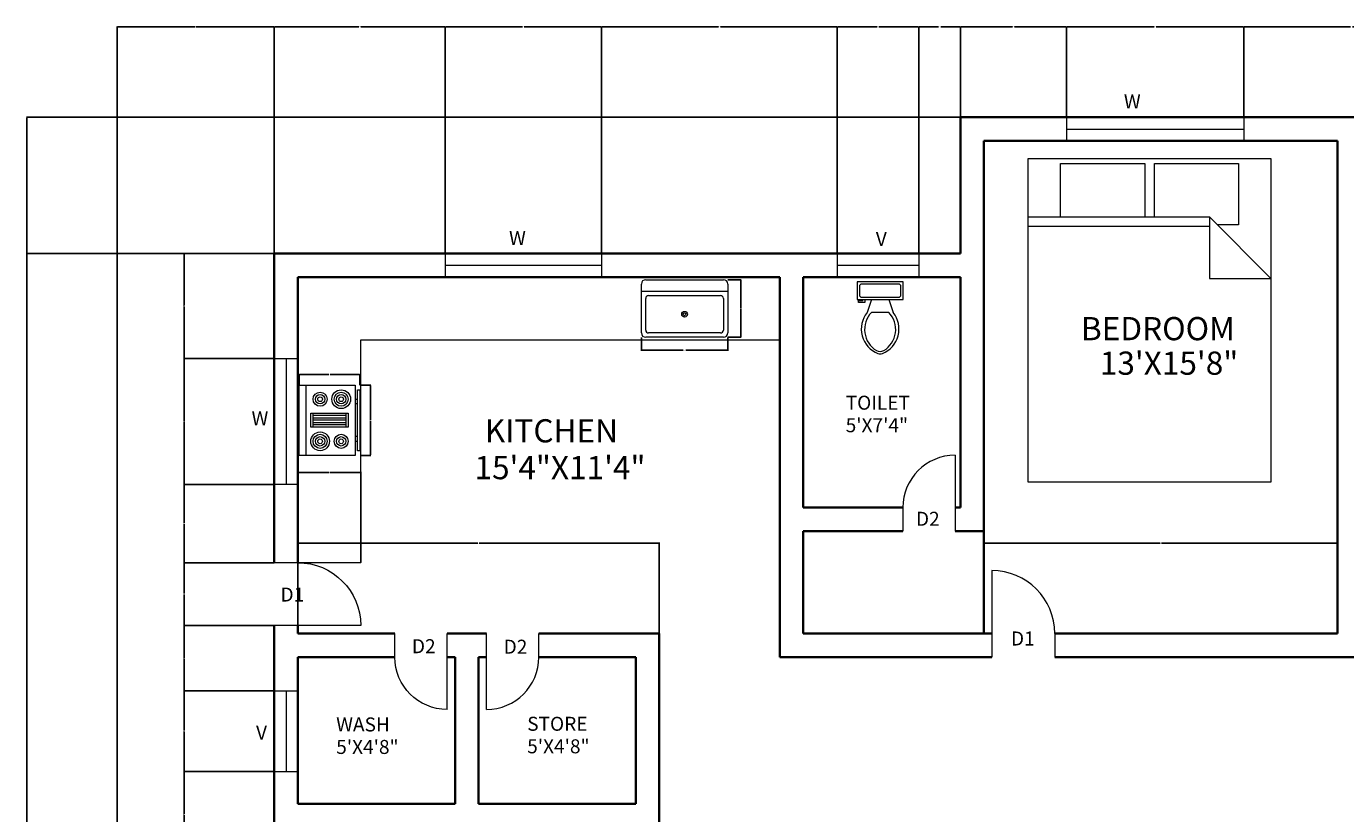
# Model space of a CAD drawing. Units: feet. Extents: x 1508 to 2265, y 1718 to 2421.
# Tile 3 of 4: x 1508 to 2012, y 2121 to 2421. Entities that reach past the tile are written whole.
import ezdxf

# ---------------------------------------------------------------- set-up
doc = ezdxf.new("R2010")
doc.units = ezdxf.units.FT
for name, color, linetype, lineweight in [('A-ANNO-DIMS', 2, 'Continuous', 18), ('A-ANNO-TEXT', 3, 'Continuous', 13), ('A-AREA-IDEN', 7, 'Continuous', 18), ('A-DOOR', 3, 'Continuous', 18), ('A-EQPM', 8, 'Continuous', 18), ('A-FLOR-CASE', 8, 'Continuous', 18), ('A-FLOR-FIXT', 9, 'Continuous', 18), ('A-FURN', 8, 'Continuous', 18), ('A-GLAZ', 4, 'Continuous', 18), ('A-WALL', 7, 'Continuous', 35), ('C-PROP', 7, 'Continuous', 25)]:
    doc.layers.add(name, color=color, linetype=linetype, lineweight=lineweight)
doc.styles.get("Standard").update_dxf_attribs({"font": 'arial.ttf'})
doc.dimstyles.get("Standard").update_dxf_attribs({"dimtxt": 0.18, "dimasz": 0.18, "dimexe": 0.18, "dimexo": 0.0625, "dimgap": 0.09, "dimtad": 0, "dimtih": 1, "dimtoh": 1, "dimdec": 4, "dimzin": 0, "dimdsep": 46, "dimtxsty": 'Standard', "dimcen": 0.09, "dimadec": 0, "dimazin": 0, "dimtfac": 1, "dimtdec": 4, "dimtofl": 0, "dimtmove": 0, "dimatfit": 3, "dimfxl": 1, "dimtolj": 1, "dimtzin": 0, "dimarcsym": 0})

# ---------------------------------------------------------------- blocks, each defined once
blk = doc.blocks.new('Toilet - top')
for p, q in [((9.5, -6), (9.5, -2)), ((-10, -8.5), (-8, -8.5)), ((-10, -9.5), (-10, -8.5)), ((-7, -9.5), (-10, -9.5)), ((-8, -8.5), (-8, -8)), ((-7, -8), (-7, -9.5)), ((-4, -8), (-6, -14)), ((4, -8), (6, -14)), ((4, -14), (-4, -14))]:
    blk.add_line(p, q)
blk.add_lwpolyline([(10.5, -8), (10.5, 0), (-10.5, 0), (-10.5, -8)], close=True)
for points in [[(-9.5, -2), (-9.5, -6)], [(8.5, -1), (-8.5, -1)], [(-8.5, -7), (8.5, -7)]]:
    blk.add_lwpolyline(points)
for centre, radius, start, end in [((-8.62, -1.88), 0.884, 81.8699, 188.1301), ((-8.62, -6.12), 0.884, 171.8699, 278.1301), ((8.62, -1.88), 0.884, 351.8699, 98.1301), ((8.62, -6.12), 0.884, 261.8699, 8.1301), ((3.52, -21.58), 12.17, 141.46911, 247.97143), ((4.2, -21.82), 11.33, 136.36773, 238.94682), ((-3.52, -21.58), 12.17, 292.02843, 38.53071), ((-4.2, -21.82), 11.33, 301.05301, 43.63209), ((0, -27.88), 4, 245.73182, 294.26817), ((0, -29), 4, 254.86053, 285.13947)]:
    blk.add_arc(centre, radius, start, end)
blk = doc.blocks.new('Range-Oven - 30 in top')
for p, q in [((0, -3), (30, -3)), ((12, -6), (18, -6)), ((13, -20), (13, -6)), ((14, -6), (14, -20)), ((15, -20), (15, -6)), ((16, -6), (16, -20)), ((17, -20), (17, -6)), ((18, -20), (12, -20)), ((6, -24), (6, -25)), ((8, -25), (8, -24)), ((22, -25), (22, -24)), ((24, -24), (24, -25))]:
    blk.add_line(p, q)
for points in [[(0, -24), (0, 0), (30, 0), (30, -24)], [(12, -21), (12, -5), (18, -5), (18, -21)], [(2, -26), (2, -25), (28, -25), (28, -26)]]:
    blk.add_lwpolyline(points, close=True)
for centre, radius in [((6, -9), 4), ((6, -9), 3), ((6, -9), 2), ((6, -9), 1), ((24, -9), 3), ((24, -9), 2), ((24, -9), 1), ((6, -18), 3), ((6, -18), 2), ((24, -18), 4), ((24, -18), 3), ((24, -18), 2), ((6, -18), 1), ((24, -18), 1)]:
    blk.add_circle(centre, radius)
blk = doc.blocks.new('Sink-single - 30 in top')
blk.add_line((-15, -3.999996), (15, -3.999996))
for points in [[(-13.5, 0), (13.5, 0)], [(-15, -18.499996), (-15, -1.5)], [(15, -1.5), (15, -18.499996)], [(-13.5, -17.499996), (-13.5, -6.499996)], [(-12.5, -5.499996), (12.5, -5.499996)], [(13.5, -6.499996), (13.5, -17.499996)], [(13.5, -19.999996), (-13.5, -19.999996)], [(12.5, -18.499996), (-12.5, -18.499996)]]:
    blk.add_lwpolyline(points)
for radius in [1, 0.5]:
    blk.add_circle((0, -11.999996), radius)
for centre, radius, start, end in [((-13.5, -1.5), 1.5, 90, 180), ((13.5, -1.5), 1.5, 0, 90), ((-12.5, -6.499996), 1, 90, 180), ((12.5, -6.499996), 1, 0, 90), ((-12.5, -17.499996), 1, 180, 270), ((12.5, -17.499996), 1, 270, 0), ((-13.5, -18.499996), 1.5, 180, 270), ((13.5, -18.499996), 1.5, 270, 0)]:
    blk.add_arc(centre, radius, start, end)
blk = doc.blocks.new('Bed - Queen')
for p, q in [((0, -80.00003), (0, 0)), ((0, 0), (59.99999, 0)), ((59.99999, 0), (59.99999, -80.00003)), ((7.99999, -1.2), (28.79998, -1.2)), ((7.99999, -14.4), (7.99999, -1.2)), ((28.79998, -1.2), (28.79998, -14.4)), ((31.19999, -1.2), (51.99999, -1.2)), ((31.19999, -14.4), (31.19999, -1.2)), ((51.99999, -1.2), (51.99999, -16.4)), ((0, -14.4), (44.8, -14.4)), ((59.99999, -29.6), (44.8, -14.4)), ((44.8, -14.4), (44.8, -29.6)), ((44.8, -16.8), (0, -16.8)), ((51.99999, -16.4), (46.79936, -16.4)), ((44.8, -29.6), (59.99999, -29.6)), ((59.99999, -80.00003), (0, -80.00003))]:
    blk.add_line(p, q)
blk = doc.blocks.new('DOOR-LEAF-24')
blk.add_line((0, 33), (0, 0))
blk.add_arc((0, 9), 24, 0, 90)
blk = doc.blocks.new('DOOR-LEAF-20')
blk.add_line((20, 29), (20, 0))
blk.add_arc((20, 9), 20, 90, 180)
blk = doc.blocks.new('*D27')
at = {"layer": 'A-ANNO-DIMS', "color": 0, "lineweight": -2, "transparency": 16777216}
for p, q in [((1635.54, 2284), (1639.67, 2284)), ((1639.49, 2283.82), (1639.49, 2270.79)), ((1639.49, 2257.39), (1639.49, 2270.42)), ((1635.54, 2257.21), (1639.67, 2257.21))]:
    blk.add_line(p, q, dxfattribs=at)
at = {"layer": 'A-ANNO-DIMS', "color": 0, "transparency": 16777216}
for points in [[(1639.46, 2283.82), (1639.52, 2283.82), (1639.49, 2284)], [(1639.46, 2257.39), (1639.52, 2257.39), (1639.49, 2257.21)]]:
    blk.add_solid(points, dxfattribs=at)
at = {"layer": 'Defpoints', "color": 0, "transparency": 16777216}
for p in [(1635.48, 2284), (1639.49, 2284), (1635.48, 2257.21)]:
    blk.add_point(p, dxfattribs=at)
at = {"layer": 'A-ANNO-DIMS', "color": 0, "transparency": 16777216, "insert": (1639.49, 2270.61), "char_height": 0.18, "attachment_point": 5}
blk.add_mtext('\\A1;RANGE 27', dxfattribs=at)
blk = doc.blocks.new('*D28')
at = {"layer": 'A-ANNO-DIMS', "color": 0, "lineweight": -2, "transparency": 16777216}
for p, q in [((1612.26, 2284.06), (1612.26, 2288.2)), ((1612.44, 2288.02), (1623.65, 2288.02)), ((1635.3, 2288.02), (1624.09, 2288.02)), ((1635.48, 2284.06), (1635.48, 2288.2))]:
    blk.add_line(p, q, dxfattribs=at)
at = {"layer": 'A-ANNO-DIMS', "color": 0, "transparency": 16777216}
for points in [[(1612.44, 2288.05), (1612.44, 2287.99), (1612.26, 2288.02)], [(1635.3, 2288.05), (1635.3, 2287.99), (1635.48, 2288.02)]]:
    blk.add_solid(points, dxfattribs=at)
at = {"layer": 'Defpoints', "color": 0, "transparency": 16777216}
for p in [(1612.26, 2288.02), (1612.26, 2284), (1635.48, 2284)]:
    blk.add_point(p, dxfattribs=at)
at = {"layer": 'A-ANNO-DIMS', "color": 0, "transparency": 16777216, "insert": (1623.87, 2288.02), "char_height": 0.18, "attachment_point": 5}
blk.add_mtext('\\A1;23', dxfattribs=at)
blk = doc.blocks.new('*D29')
at = {"layer": 'A-ANNO-DIMS', "color": 0, "lineweight": -2, "transparency": 16777216}
for p, q in [((1742.98, 2302.21), (1742.98, 2297.15)), ((1743.16, 2297.33), (1758.92, 2297.33)), ((1775.77, 2297.33), (1760.01, 2297.33)), ((1775.95, 2302.21), (1775.95, 2297.15))]:
    blk.add_line(p, q, dxfattribs=at)
at = {"layer": 'A-ANNO-DIMS', "color": 0, "transparency": 16777216}
for points in [[(1743.16, 2297.36), (1743.16, 2297.3), (1742.98, 2297.33)], [(1775.77, 2297.36), (1775.77, 2297.3), (1775.95, 2297.33)]]:
    blk.add_solid(points, dxfattribs=at)
at = {"layer": 'Defpoints', "color": 0, "transparency": 16777216}
for p in [(1742.98, 2302.28), (1775.95, 2302.28), (1775.95, 2297.33)]:
    blk.add_point(p, dxfattribs=at)
at = {"layer": 'A-ANNO-DIMS', "color": 0, "transparency": 16777216, "insert": (1759.46, 2297.33), "char_height": 0.18, "attachment_point": 5}
blk.add_mtext('\\A1;SINK 33', dxfattribs=at)
blk = doc.blocks.new('*D30')
at = {"layer": 'A-ANNO-DIMS', "color": 0, "lineweight": -2, "transparency": 16777216}
for p, q in [((1776.01, 2324.26), (1781.08, 2324.26)), ((1780.9, 2324.08), (1780.9, 2313.45)), ((1780.9, 2302.46), (1780.9, 2313.09)), ((1776.01, 2302.28), (1781.08, 2302.28))]:
    blk.add_line(p, q, dxfattribs=at)
at = {"layer": 'A-ANNO-DIMS', "color": 0, "transparency": 16777216}
for points in [[(1780.87, 2324.08), (1780.93, 2324.08), (1780.9, 2324.26)], [(1780.87, 2302.46), (1780.93, 2302.46), (1780.9, 2302.28)]]:
    blk.add_solid(points, dxfattribs=at)
at = {"layer": 'Defpoints', "color": 0, "transparency": 16777216}
for p in [(1775.95, 2324.26), (1780.9, 2324.26), (1775.95, 2302.28)]:
    blk.add_point(p, dxfattribs=at)
at = {"layer": 'A-ANNO-DIMS', "color": 0, "transparency": 16777216, "insert": (1780.9, 2313.27), "char_height": 0.18, "attachment_point": 5}
blk.add_mtext('\\A1;22', dxfattribs=at)
blk = doc.blocks.new('*D32')
at = {"layer": 'A-ANNO-DIMS', "color": 0, "lineweight": -2, "transparency": 16777216}
for p, q in [((1542.74, 2386.26), (1508.15, 2386.26)), ((1508.33, 2386.08), (1508.33, 2069.44)), ((1508.33, 1752.44), (1508.33, 2069.08)), ((1542.74, 1752.26), (1508.15, 1752.26))]:
    blk.add_line(p, q, dxfattribs=at)
at = {"layer": 'A-ANNO-DIMS', "color": 0, "transparency": 16777216}
for points in [[(1508.3, 2386.08), (1508.36, 2386.08), (1508.33, 2386.26)], [(1508.3, 1752.44), (1508.36, 1752.44), (1508.33, 1752.26)]]:
    blk.add_solid(points, dxfattribs=at)
at = {"layer": 'Defpoints', "color": 0, "transparency": 16777216}
for p in [(1508.33, 2386.26), (1542.8, 2386.26), (1542.8, 1752.26)]:
    blk.add_point(p, dxfattribs=at)
at = {"layer": 'A-ANNO-DIMS', "color": 0, "transparency": 16777216, "insert": (1508.33, 2069.26), "char_height": 0.18, "attachment_point": 5}
blk.add_mtext('\\A1;634', dxfattribs=at)
blk = doc.blocks.new('*D33')
at = {"layer": 'A-ANNO-DIMS', "color": 0, "lineweight": -2, "transparency": 16777216}
for p, q in [((1542.8, 2386.32), (1542.8, 2420.92)), ((1542.98, 2420.74), (1572.59, 2420.74)), ((1602.62, 2420.74), (1573.02, 2420.74)), ((1602.8, 2334.32), (1602.8, 2420.92))]:
    blk.add_line(p, q, dxfattribs=at)
at = {"layer": 'A-ANNO-DIMS', "color": 0, "transparency": 16777216}
for points in [[(1542.98, 2420.77), (1542.98, 2420.71), (1542.8, 2420.74)], [(1602.62, 2420.77), (1602.62, 2420.71), (1602.8, 2420.74)]]:
    blk.add_solid(points, dxfattribs=at)
at = {"layer": 'Defpoints', "color": 0, "transparency": 16777216}
for p in [(1602.8, 2420.74), (1542.8, 2386.26), (1602.8, 2334.26)]:
    blk.add_point(p, dxfattribs=at)
at = {"layer": 'A-ANNO-DIMS', "color": 0, "transparency": 16777216, "insert": (1572.8, 2420.74), "char_height": 0.18, "attachment_point": 5}
blk.add_mtext('\\A1;60', dxfattribs=at)
blk = doc.blocks.new('*D36')
at = {"layer": 'A-ANNO-DIMS', "color": 0, "lineweight": -2, "transparency": 16777216}
for p, q in [((1864.74, 2386.26), (1508.15, 2386.26)), ((1508.33, 2386.08), (1508.33, 2360.44)), ((1508.33, 2334.44), (1508.33, 2360.08)), ((1864.74, 2334.26), (1508.15, 2334.26))]:
    blk.add_line(p, q, dxfattribs=at)
at = {"layer": 'A-ANNO-DIMS', "color": 0, "transparency": 16777216}
for points in [[(1508.3, 2386.08), (1508.36, 2386.08), (1508.33, 2386.26)], [(1508.3, 2334.44), (1508.36, 2334.44), (1508.33, 2334.26)]]:
    blk.add_solid(points, dxfattribs=at)
at = {"layer": 'Defpoints', "color": 0, "transparency": 16777216}
for p in [(1508.33, 2386.26), (1864.8, 2386.26), (1864.8, 2334.26)]:
    blk.add_point(p, dxfattribs=at)
at = {"layer": 'A-ANNO-DIMS', "color": 0, "transparency": 16777216, "insert": (1508.33, 2360.26), "char_height": 0.18, "attachment_point": 5}
blk.add_mtext('\\A1;52', dxfattribs=at)
blk = doc.blocks.new('*D37')
at = {"layer": 'A-ANNO-DIMS', "color": 0, "lineweight": -2, "transparency": 16777216}
for p, q in [((1602.8, 2334.32), (1602.8, 2420.92)), ((1602.98, 2420.74), (1635.05, 2420.74)), ((1667.91, 2420.74), (1635.84, 2420.74)), ((1668.09, 2334.32), (1668.09, 2420.92))]:
    blk.add_line(p, q, dxfattribs=at)
at = {"layer": 'A-ANNO-DIMS', "color": 0, "transparency": 16777216}
for points in [[(1602.98, 2420.77), (1602.98, 2420.71), (1602.8, 2420.74)], [(1667.91, 2420.77), (1667.91, 2420.71), (1668.09, 2420.74)]]:
    blk.add_solid(points, dxfattribs=at)
at = {"layer": 'Defpoints', "color": 0, "transparency": 16777216}
for p in [(1668.09, 2420.74), (1602.8, 2334.26), (1668.09, 2334.26)]:
    blk.add_point(p, dxfattribs=at)
at = {"layer": 'A-ANNO-DIMS', "color": 0, "transparency": 16777216, "insert": (1635.45, 2420.74), "char_height": 0.18, "attachment_point": 5}
blk.add_mtext('\\A1;65.29', dxfattribs=at)
blk = doc.blocks.new('*D38')
at = {"layer": 'A-ANNO-DIMS', "color": 0, "lineweight": -2, "transparency": 16777216}
for p, q in [((1668.09, 2334.32), (1668.09, 2420.92)), ((1668.27, 2420.74), (1697.62, 2420.74)), ((1727.61, 2420.74), (1698.27, 2420.74)), ((1727.79, 2334.32), (1727.79, 2420.92))]:
    blk.add_line(p, q, dxfattribs=at)
at = {"layer": 'A-ANNO-DIMS', "color": 0, "transparency": 16777216}
for points in [[(1668.27, 2420.77), (1668.27, 2420.71), (1668.09, 2420.74)], [(1727.61, 2420.77), (1727.61, 2420.71), (1727.79, 2420.74)]]:
    blk.add_solid(points, dxfattribs=at)
at = {"layer": 'Defpoints', "color": 0, "transparency": 16777216}
for p in [(1727.79, 2420.74), (1668.09, 2334.26), (1727.79, 2334.26)]:
    blk.add_point(p, dxfattribs=at)
at = {"layer": 'A-ANNO-DIMS', "color": 0, "transparency": 16777216, "insert": (1697.94, 2420.74), "char_height": 0.18, "attachment_point": 5}
blk.add_mtext('\\A1;59.7', dxfattribs=at)
blk = doc.blocks.new('*D39')
at = {"layer": 'A-ANNO-DIMS', "color": 0, "lineweight": -2, "transparency": 16777216}
for p, q in [((1727.79, 2334.32), (1727.79, 2420.92)), ((1727.97, 2420.74), (1772.39, 2420.74)), ((1817.6, 2420.74), (1773.18, 2420.74)), ((1817.78, 2334.32), (1817.78, 2420.92))]:
    blk.add_line(p, q, dxfattribs=at)
at = {"layer": 'A-ANNO-DIMS', "color": 0, "transparency": 16777216}
for points in [[(1727.97, 2420.77), (1727.97, 2420.71), (1727.79, 2420.74)], [(1817.6, 2420.77), (1817.6, 2420.71), (1817.78, 2420.74)]]:
    blk.add_solid(points, dxfattribs=at)
at = {"layer": 'Defpoints', "color": 0, "transparency": 16777216}
for p in [(1817.78, 2420.74), (1727.79, 2334.26), (1817.78, 2334.26)]:
    blk.add_point(p, dxfattribs=at)
at = {"layer": 'A-ANNO-DIMS', "color": 0, "transparency": 16777216, "insert": (1772.79, 2420.74), "char_height": 0.18, "attachment_point": 5}
blk.add_mtext('\\A1;89.98', dxfattribs=at)
blk = doc.blocks.new('*D40')
at = {"layer": 'A-ANNO-DIMS', "color": 0, "lineweight": -2, "transparency": 16777216}
for p, q in [((1817.78, 2334.32), (1817.78, 2420.92)), ((1817.96, 2420.74), (1833.02, 2420.74)), ((1848.7, 2420.74), (1833.63, 2420.74)), ((1848.88, 2334.32), (1848.88, 2420.92))]:
    blk.add_line(p, q, dxfattribs=at)
at = {"layer": 'A-ANNO-DIMS', "color": 0, "transparency": 16777216}
for points in [[(1817.96, 2420.77), (1817.96, 2420.71), (1817.78, 2420.74)], [(1848.7, 2420.77), (1848.7, 2420.71), (1848.88, 2420.74)]]:
    blk.add_solid(points, dxfattribs=at)
at = {"layer": 'Defpoints', "color": 0, "transparency": 16777216}
for p in [(1848.88, 2420.74), (1817.78, 2334.26), (1848.88, 2334.26)]:
    blk.add_point(p, dxfattribs=at)
at = {"layer": 'A-ANNO-DIMS', "color": 0, "transparency": 16777216, "insert": (1833.33, 2420.74), "char_height": 0.18, "attachment_point": 5}
blk.add_mtext('\\A1;31.1', dxfattribs=at)
blk = doc.blocks.new('*D41')
at = {"layer": 'A-ANNO-DIMS', "color": 0, "lineweight": -2, "transparency": 16777216}
for p, q in [((1848.88, 2334.32), (1848.88, 2420.92)), ((1849.06, 2420.74), (1856.39, 2420.74)), ((1864.62, 2420.74), (1857.3, 2420.74)), ((1864.8, 2334.32), (1864.8, 2420.92))]:
    blk.add_line(p, q, dxfattribs=at)
at = {"layer": 'A-ANNO-DIMS', "color": 0, "transparency": 16777216}
for points in [[(1849.06, 2420.77), (1849.06, 2420.71), (1848.88, 2420.74)], [(1864.62, 2420.77), (1864.62, 2420.71), (1864.8, 2420.74)]]:
    blk.add_solid(points, dxfattribs=at)
at = {"layer": 'Defpoints', "color": 0, "transparency": 16777216}
for p in [(1864.8, 2420.74), (1848.88, 2334.26), (1864.8, 2334.26)]:
    blk.add_point(p, dxfattribs=at)
at = {"layer": 'A-ANNO-DIMS', "color": 0, "transparency": 16777216, "insert": (1856.84, 2420.74), "char_height": 0.18, "attachment_point": 5}
blk.add_mtext('\\A1;15.928', dxfattribs=at)
blk = doc.blocks.new('*D42')
at = {"layer": 'A-ANNO-DIMS', "color": 0, "lineweight": -2, "transparency": 16777216}
for p, q in [((1864.8, 2386.32), (1864.8, 2420.92)), ((1864.98, 2420.74), (1884.69, 2420.74)), ((1905.18, 2420.74), (1885.48, 2420.74)), ((1905.36, 2386.32), (1905.36, 2420.92))]:
    blk.add_line(p, q, dxfattribs=at)
at = {"layer": 'A-ANNO-DIMS', "color": 0, "transparency": 16777216}
for points in [[(1864.98, 2420.77), (1864.98, 2420.71), (1864.8, 2420.74)], [(1905.18, 2420.77), (1905.18, 2420.71), (1905.36, 2420.74)]]:
    blk.add_solid(points, dxfattribs=at)
at = {"layer": 'Defpoints', "color": 0, "transparency": 16777216}
for p in [(1905.36, 2420.74), (1864.8, 2386.26), (1905.36, 2386.26)]:
    blk.add_point(p, dxfattribs=at)
at = {"layer": 'A-ANNO-DIMS', "color": 0, "transparency": 16777216, "insert": (1885.08, 2420.74), "char_height": 0.18, "attachment_point": 5}
blk.add_mtext('\\A1;40.56', dxfattribs=at)
blk = doc.blocks.new('*D43')
at = {"layer": 'A-ANNO-DIMS', "color": 0, "lineweight": -2, "transparency": 16777216}
for p, q in [((1905.36, 2386.32), (1905.36, 2420.92)), ((1905.54, 2420.74), (1938.79, 2420.74)), ((1972.79, 2420.74), (1939.54, 2420.74)), ((1972.97, 2386.32), (1972.97, 2420.92))]:
    blk.add_line(p, q, dxfattribs=at)
at = {"layer": 'A-ANNO-DIMS', "color": 0, "transparency": 16777216}
for points in [[(1905.54, 2420.77), (1905.54, 2420.71), (1905.36, 2420.74)], [(1972.79, 2420.77), (1972.79, 2420.71), (1972.97, 2420.74)]]:
    blk.add_solid(points, dxfattribs=at)
at = {"layer": 'Defpoints', "color": 0, "transparency": 16777216}
for p in [(1972.97, 2420.74), (1905.36, 2386.26), (1972.97, 2386.26)]:
    blk.add_point(p, dxfattribs=at)
at = {"layer": 'A-ANNO-DIMS', "color": 0, "transparency": 16777216, "insert": (1939.17, 2420.74), "char_height": 0.18, "attachment_point": 5}
blk.add_mtext('\\A1;67.61', dxfattribs=at)
blk = doc.blocks.new('*D44')
at = {"layer": 'A-ANNO-DIMS', "color": 0, "lineweight": -2, "transparency": 16777216}
for p, q in [((1972.97, 2386.32), (1972.97, 2420.92)), ((1973.15, 2420.74), (2013.79, 2420.74)), ((2055.22, 2420.74), (2014.58, 2420.74)), ((2055.4, 2386.32), (2055.4, 2420.92))]:
    blk.add_line(p, q, dxfattribs=at)
at = {"layer": 'A-ANNO-DIMS', "color": 0, "transparency": 16777216}
for points in [[(1973.15, 2420.77), (1973.15, 2420.71), (1972.97, 2420.74)], [(2055.22, 2420.77), (2055.22, 2420.71), (2055.4, 2420.74)]]:
    blk.add_solid(points, dxfattribs=at)
at = {"layer": 'Defpoints', "color": 0, "transparency": 16777216}
for p in [(2055.4, 2420.74), (1972.97, 2386.26), (2055.4, 2386.26)]:
    blk.add_point(p, dxfattribs=at)
at = {"layer": 'A-ANNO-DIMS', "color": 0, "transparency": 16777216, "insert": (2014.19, 2420.74), "char_height": 0.18, "attachment_point": 5}
blk.add_mtext('\\A1;82.43', dxfattribs=at)
blk = doc.blocks.new('*D59')
at = {"layer": 'A-ANNO-DIMS', "color": 0, "lineweight": -2, "transparency": 16777216}
for p, q in [((1602.74, 2136.59), (1568.15, 2136.59)), ((1568.33, 2136.41), (1568.33, 2120.4)), ((1568.33, 2104.02), (1568.33, 2120.03)), ((1602.74, 2103.84), (1568.15, 2103.84))]:
    blk.add_line(p, q, dxfattribs=at)
at = {"layer": 'A-ANNO-DIMS', "color": 0, "transparency": 16777216}
for points in [[(1568.3, 2136.41), (1568.36, 2136.41), (1568.33, 2136.59)], [(1568.3, 2104.02), (1568.36, 2104.02), (1568.33, 2103.84)]]:
    blk.add_solid(points, dxfattribs=at)
at = {"layer": 'Defpoints', "color": 0, "transparency": 16777216}
for p in [(1568.33, 2136.59), (1602.8, 2136.59), (1602.8, 2103.84)]:
    blk.add_point(p, dxfattribs=at)
at = {"layer": 'A-ANNO-DIMS', "color": 0, "transparency": 16777216, "insert": (1568.33, 2120.22), "char_height": 0.18, "attachment_point": 5}
blk.add_mtext('\\A1;32.74', dxfattribs=at)
blk = doc.blocks.new('*D60')
at = {"layer": 'A-ANNO-DIMS', "color": 0, "lineweight": -2, "transparency": 16777216}
for p, q in [((1602.74, 2167.39), (1568.15, 2167.39)), ((1568.33, 2167.21), (1568.33, 2152.17)), ((1568.33, 2136.77), (1568.33, 2151.81)), ((1602.74, 2136.59), (1568.15, 2136.59))]:
    blk.add_line(p, q, dxfattribs=at)
at = {"layer": 'A-ANNO-DIMS', "color": 0, "transparency": 16777216}
for points in [[(1568.3, 2167.21), (1568.36, 2167.21), (1568.33, 2167.39)], [(1568.3, 2136.77), (1568.36, 2136.77), (1568.33, 2136.59)]]:
    blk.add_solid(points, dxfattribs=at)
at = {"layer": 'Defpoints', "color": 0, "transparency": 16777216}
for p in [(1568.33, 2167.39), (1602.8, 2167.39), (1602.8, 2136.59)]:
    blk.add_point(p, dxfattribs=at)
at = {"layer": 'A-ANNO-DIMS', "color": 0, "transparency": 16777216, "insert": (1568.33, 2151.99), "char_height": 0.18, "attachment_point": 5}
blk.add_mtext('\\A1;30.803', dxfattribs=at)
blk = doc.blocks.new('*D61')
at = {"layer": 'A-ANNO-DIMS', "color": 0, "lineweight": -2, "transparency": 16777216}
for p, q in [((1602.74, 2192.26), (1568.15, 2192.26)), ((1568.33, 2192.08), (1568.33, 2180.01)), ((1568.33, 2167.57), (1568.33, 2179.64)), ((1602.74, 2167.39), (1568.15, 2167.39))]:
    blk.add_line(p, q, dxfattribs=at)
at = {"layer": 'A-ANNO-DIMS', "color": 0, "transparency": 16777216}
for points in [[(1568.3, 2192.08), (1568.36, 2192.08), (1568.33, 2192.26)], [(1568.3, 2167.57), (1568.36, 2167.57), (1568.33, 2167.39)]]:
    blk.add_solid(points, dxfattribs=at)
at = {"layer": 'Defpoints', "color": 0, "transparency": 16777216}
for p in [(1568.33, 2192.26), (1602.8, 2192.26), (1602.8, 2167.39)]:
    blk.add_point(p, dxfattribs=at)
at = {"layer": 'A-ANNO-DIMS', "color": 0, "transparency": 16777216, "insert": (1568.33, 2179.83), "char_height": 0.18, "attachment_point": 5}
blk.add_mtext('\\A1;24.87', dxfattribs=at)
blk = doc.blocks.new('*D62')
at = {"layer": 'A-ANNO-DIMS', "color": 0, "lineweight": -2, "transparency": 16777216}
for p, q in [((1602.74, 2216.26), (1568.15, 2216.26)), ((1568.33, 2216.08), (1568.33, 2204.44)), ((1568.33, 2192.44), (1568.33, 2204.08)), ((1602.74, 2192.26), (1568.15, 2192.26))]:
    blk.add_line(p, q, dxfattribs=at)
at = {"layer": 'A-ANNO-DIMS', "color": 0, "transparency": 16777216}
for points in [[(1568.3, 2216.08), (1568.36, 2216.08), (1568.33, 2216.26)], [(1568.3, 2192.44), (1568.36, 2192.44), (1568.33, 2192.26)]]:
    blk.add_solid(points, dxfattribs=at)
at = {"layer": 'Defpoints', "color": 0, "transparency": 16777216}
for p in [(1568.33, 2216.26), (1602.8, 2216.26), (1602.8, 2192.26)]:
    blk.add_point(p, dxfattribs=at)
at = {"layer": 'A-ANNO-DIMS', "color": 0, "transparency": 16777216, "insert": (1568.33, 2204.26), "char_height": 0.18, "attachment_point": 5}
blk.add_mtext('\\A1;24', dxfattribs=at)
blk = doc.blocks.new('*D63')
at = {"layer": 'A-ANNO-DIMS', "color": 0, "lineweight": -2, "transparency": 16777216}
for p, q in [((1602.74, 2246.14), (1568.15, 2246.14)), ((1568.33, 2245.96), (1568.33, 2231.38)), ((1568.33, 2216.44), (1568.33, 2231.02)), ((1602.74, 2216.26), (1568.15, 2216.26))]:
    blk.add_line(p, q, dxfattribs=at)
at = {"layer": 'A-ANNO-DIMS', "color": 0, "transparency": 16777216}
for points in [[(1568.3, 2245.96), (1568.36, 2245.96), (1568.33, 2246.14)], [(1568.3, 2216.44), (1568.36, 2216.44), (1568.33, 2216.26)]]:
    blk.add_solid(points, dxfattribs=at)
at = {"layer": 'Defpoints', "color": 0, "transparency": 16777216}
for p in [(1568.33, 2246.14), (1602.8, 2246.14), (1602.8, 2216.26)]:
    blk.add_point(p, dxfattribs=at)
at = {"layer": 'A-ANNO-DIMS', "color": 0, "transparency": 16777216, "insert": (1568.33, 2231.2), "char_height": 0.18, "attachment_point": 5}
blk.add_mtext('\\A1;29.88', dxfattribs=at)
blk = doc.blocks.new('*D64')
at = {"layer": 'A-ANNO-DIMS', "color": 0, "lineweight": -2, "transparency": 16777216}
for p, q in [((1602.74, 2294.14), (1568.15, 2294.14)), ((1568.33, 2293.96), (1568.33, 2270.32)), ((1568.33, 2246.32), (1568.33, 2269.96)), ((1602.74, 2246.14), (1568.15, 2246.14))]:
    blk.add_line(p, q, dxfattribs=at)
at = {"layer": 'A-ANNO-DIMS', "color": 0, "transparency": 16777216}
for points in [[(1568.3, 2293.96), (1568.36, 2293.96), (1568.33, 2294.14)], [(1568.3, 2246.32), (1568.36, 2246.32), (1568.33, 2246.14)]]:
    blk.add_solid(points, dxfattribs=at)
at = {"layer": 'Defpoints', "color": 0, "transparency": 16777216}
for p in [(1568.33, 2294.14), (1602.8, 2294.14), (1602.8, 2246.14)]:
    blk.add_point(p, dxfattribs=at)
at = {"layer": 'A-ANNO-DIMS', "color": 0, "transparency": 16777216, "insert": (1568.33, 2270.14), "char_height": 0.18, "attachment_point": 5}
blk.add_mtext('\\A1;48', dxfattribs=at)
blk = doc.blocks.new('*D65')
at = {"layer": 'A-ANNO-DIMS', "color": 0, "lineweight": -2, "transparency": 16777216}
for p, q in [((1602.74, 2334.26), (1568.15, 2334.26)), ((1568.33, 2334.08), (1568.33, 2314.38)), ((1568.33, 2294.32), (1568.33, 2314.02)), ((1602.74, 2294.14), (1568.15, 2294.14))]:
    blk.add_line(p, q, dxfattribs=at)
at = {"layer": 'A-ANNO-DIMS', "color": 0, "transparency": 16777216}
for points in [[(1568.3, 2334.08), (1568.36, 2334.08), (1568.33, 2334.26)], [(1568.3, 2294.32), (1568.36, 2294.32), (1568.33, 2294.14)]]:
    blk.add_solid(points, dxfattribs=at)
at = {"layer": 'Defpoints', "color": 0, "transparency": 16777216}
for p in [(1568.33, 2334.26), (1602.8, 2334.26), (1602.8, 2294.14)]:
    blk.add_point(p, dxfattribs=at)
at = {"layer": 'A-ANNO-DIMS', "color": 0, "transparency": 16777216, "insert": (1568.33, 2314.2), "char_height": 0.18, "attachment_point": 5}
blk.add_mtext('\\A1;40.12', dxfattribs=at)
blk = doc.blocks.new('*D80')
at = {"layer": 'A-ANNO-DIMS', "color": 0, "lineweight": -2, "transparency": 16777216}
for p, q in [((1873.8, 2189.32), (1873.8, 2223.92)), ((1873.98, 2223.74), (1941.02, 2223.74)), ((2008.62, 2223.74), (1941.59, 2223.74)), ((2008.8, 2189.32), (2008.8, 2223.92))]:
    blk.add_line(p, q, dxfattribs=at)
at = {"layer": 'A-ANNO-DIMS', "color": 0, "transparency": 16777216}
for points in [[(1873.98, 2223.77), (1873.98, 2223.71), (1873.8, 2223.74)], [(2008.62, 2223.77), (2008.62, 2223.71), (2008.8, 2223.74)]]:
    blk.add_solid(points, dxfattribs=at)
at = {"layer": 'Defpoints', "color": 0, "transparency": 16777216}
for p in [(2008.8, 2223.74), (1873.8, 2189.26), (2008.8, 2189.26)]:
    blk.add_point(p, dxfattribs=at)
at = {"layer": 'A-ANNO-DIMS', "color": 0, "transparency": 16777216, "insert": (1941.3, 2223.74), "char_height": 0.18, "attachment_point": 5}
blk.add_mtext('\\A1;135', dxfattribs=at)
blk = doc.blocks.new('*D81')
at = {"layer": 'A-ANNO-DIMS', "color": 0, "lineweight": -2, "transparency": 16777216}
for p, q in [((1611.8, 2189.32), (1611.8, 2223.92)), ((1611.98, 2223.74), (1680.52, 2223.74)), ((1749.62, 2223.74), (1681.09, 2223.74)), ((1749.8, 2189.32), (1749.8, 2223.92))]:
    blk.add_line(p, q, dxfattribs=at)
at = {"layer": 'A-ANNO-DIMS', "color": 0, "transparency": 16777216}
for points in [[(1611.98, 2223.77), (1611.98, 2223.71), (1611.8, 2223.74)], [(1749.62, 2223.77), (1749.62, 2223.71), (1749.8, 2223.74)]]:
    blk.add_solid(points, dxfattribs=at)
at = {"layer": 'Defpoints', "color": 0, "transparency": 16777216}
for p in [(1749.8, 2223.74), (1611.8, 2189.26), (1749.8, 2189.26)]:
    blk.add_point(p, dxfattribs=at)
at = {"layer": 'A-ANNO-DIMS', "color": 0, "transparency": 16777216, "insert": (1680.8, 2223.74), "char_height": 0.18, "attachment_point": 5}
blk.add_mtext('\\A1;138', dxfattribs=at)
blk = doc.blocks.new('*D82')
at = {"layer": 'A-ANNO-DIMS', "color": 0, "lineweight": -2, "transparency": 16777216}
for p, q in [((1611.8, 2216.32), (1611.8, 2250.92)), ((1611.98, 2250.74), (1623.58, 2250.74)), ((1635.62, 2250.74), (1624.02, 2250.74)), ((1635.8, 2216.32), (1635.8, 2250.92))]:
    blk.add_line(p, q, dxfattribs=at)
at = {"layer": 'A-ANNO-DIMS', "color": 0, "transparency": 16777216}
for points in [[(1611.98, 2250.77), (1611.98, 2250.71), (1611.8, 2250.74)], [(1635.62, 2250.77), (1635.62, 2250.71), (1635.8, 2250.74)]]:
    blk.add_solid(points, dxfattribs=at)
at = {"layer": 'Defpoints', "color": 0, "transparency": 16777216}
for p in [(1635.8, 2250.74), (1611.8, 2216.26), (1635.8, 2216.26)]:
    blk.add_point(p, dxfattribs=at)
at = {"layer": 'A-ANNO-DIMS', "color": 0, "transparency": 16777216, "insert": (1623.8, 2250.74), "char_height": 0.18, "attachment_point": 5}
blk.add_mtext('\\A1;24', dxfattribs=at)

msp = doc.modelspace()

# ---------------------------------------------------------------- linework, layer by layer
at = {"layer": 'A-DOOR'}
for p, q in [((1842.8049, 2237.2608), (1842.8049, 2228.2608)), ((1648.8049, 2180.2608), (1648.8049, 2189.2608)), ((1703.8049, 2180.2608), (1703.8049, 2189.2608)), ((1900.8049, 2189.2608), (1900.8049, 2180.2608))]:
    msp.add_line(p, q, dxfattribs=at)
at = {"layer": 'A-FLOR-CASE'}
for p, q in [((1635.8049, 2301.2608), (1795.8049, 2301.2608)), ((1635.8049, 2216.2608), (1635.8049, 2301.2608)), ((1635.8049, 2216.2608), (1602.8049, 2216.2608))]:
    msp.add_line(p, q, dxfattribs=at)
at = {"layer": 'A-GLAZ'}
for p, q in [((1905.3626, 2386.2608), (1905.3626, 2377.2608)), ((1972.9732, 2386.2608), (1972.9732, 2377.2608)), ((1905.3626, 2381.7608), (1972.9732, 2381.7608)), ((1668.0907, 2334.2608), (1668.0907, 2325.2608)), ((1727.7948, 2334.2608), (1727.7948, 2325.2608)), ((1817.7791, 2334.2608), (1817.7791, 2325.2608)), ((1848.8765, 2334.2608), (1848.8765, 2325.2608)), ((1668.0907, 2329.7608), (1727.7948, 2329.7608)), ((1817.7791, 2329.7608), (1848.8765, 2329.7608)), ((1602.8049, 2294.1395), (1611.8049, 2294.1395)), ((1607.3049, 2294.1395), (1607.3049, 2246.1395)), ((1611.8049, 2246.1395), (1602.8049, 2246.1395)), ((1602.8049, 2167.3913), (1611.8049, 2167.3913)), ((1607.3049, 2167.3913), (1607.3049, 2136.588)), ((1602.8049, 2136.588), (1611.8049, 2136.588))]:
    msp.add_line(p, q, dxfattribs=at)
at = {"layer": 'A-WALL'}
for p, q in [((2170.8049, 2386.2608), (1864.8049, 2386.2608)), ((1864.8049, 2334.2608), (1864.8049, 2386.2608)), ((1873.8049, 2377.2608), (1873.8049, 2189.2608)), ((2008.8049, 2377.2608), (1873.8049, 2377.2608)), ((2008.8049, 2377.2608), (2008.8049, 2189.2608)), ((1602.8049, 2334.2608), (1864.8049, 2334.2608)), ((1602.8049, 2334.2608), (1602.8049, 2216.2608)), ((1602.8049, 2216.2608), (1602.8049, 2334.2608)), ((1804.8049, 2334.2608), (1864.8049, 2334.2608)), ((1611.8049, 2325.2608), (1795.8049, 2325.2608)), ((1611.8049, 2216.2608), (1611.8049, 2325.2608)), ((1795.8049, 2325.2608), (1795.8049, 2180.2608)), ((1804.8049, 2325.2608), (1804.8049, 2237.2608)), ((1804.8049, 2325.2608), (1864.8049, 2325.2608)), ((1864.8049, 2325.2608), (1864.8049, 2237.2608)), ((1842.8049, 2237.2608), (1804.8049, 2237.2608)), ((1864.8049, 2237.2608), (1862.8049, 2237.2608)), ((1804.8049, 2228.2608), (1804.8049, 2189.2608)), ((1842.8049, 2228.2608), (1804.8049, 2228.2608)), ((1873.8049, 2228.2608), (1862.8049, 2228.2608)), ((1602.8049, 2189.2608), (1602.8049, 2192.2608)), ((1602.8049, 2192.2608), (1602.8049, 1752.2608)), ((1611.8049, 2189.2608), (1611.8049, 2192.2608)), ((1648.8049, 2189.2608), (1611.8049, 2189.2608)), ((1683.8049, 2189.2608), (1668.8049, 2189.2608)), ((1749.8049, 2189.2608), (1703.8049, 2189.2608)), ((1749.8049, 2189.2608), (1749.8049, 2082.2608)), ((1804.8049, 2189.2608), (1873.8049, 2189.2608)), ((1873.8049, 2189.2608), (1876.8049, 2189.2608)), ((1900.8049, 2189.2608), (2008.8049, 2189.2608)), ((1611.8049, 2180.2608), (1611.8049, 2124.2608)), ((1648.8049, 2180.2608), (1611.8049, 2180.2608)), ((1671.8049, 2180.2608), (1668.8049, 2180.2608)), ((1671.8049, 2124.2608), (1671.8049, 2180.2608)), ((1680.8049, 2124.2608), (1680.8049, 2180.2608)), ((1683.8049, 2180.2608), (1680.8049, 2180.2608)), ((1740.8049, 2180.2608), (1703.8049, 2180.2608)), ((1740.8049, 2124.2608), (1740.8049, 2180.2608)), ((1749.8049, 2124.2608), (1749.8049, 2180.2608)), ((1795.8049, 2180.2608), (1873.8049, 2180.2608)), ((1873.8049, 2180.2608), (1876.8049, 2180.2608)), ((1900.8049, 2180.2608), (2020.8049, 2180.2608)), ((1611.8049, 2124.2608), (1671.8049, 2124.2608)), ((1680.8049, 2124.2608), (1740.8049, 2124.2608))]:
    msp.add_line(p, q, dxfattribs=at)
at = {"layer": 'C-PROP'}
for p, q in [((1542.8049, 2386.2608), (1542.8049, 1752.2608)), ((1550.6008, 2386.2608), (1542.8049, 2386.2608)), ((1864.8049, 2386.2608), (1550.6008, 2386.2608))]:
    msp.add_line(p, q, dxfattribs=at)

# ---------------------------------------------------------------- block references
at = {"layer": 'A-DOOR'}
for name, p in [('DOOR-LEAF-20', (1842.805, 2228.261)), ('DOOR-LEAF-24', (1876.805, 2180.261))]:
    msp.add_blockref(name, p, dxfattribs=at)
at = {"layer": 'A-DOOR', "extrusion": (0, 0, -1), "zscale": -1}
for name, p, rotation in [('DOOR-LEAF-24', (-1602.8051, 2192.2609), 90.00000000000003), ('DOOR-LEAF-20', (-1648.805, 2189.2605), 180)]:
    msp.add_blockref(name, p, dxfattribs=dict(at, rotation=rotation))
at = {"layer": 'A-DOOR', "rotation": 180}
msp.add_blockref('DOOR-LEAF-20', (1703.8048, 2189.2605), dxfattribs=at)
at = {"layer": 'A-EQPM', "xscale": 0.8928425473351428, "yscale": 0.8928425473351428, "zscale": 0.8928425473351428, "rotation": 90}
msp.add_blockref('Range-Oven - 30 in top', (1612.2625, 2257.2143), dxfattribs=at)
at = {"layer": 'A-FLOR-FIXT'}
for name, p, xscale, yscale, zscale in [('Sink-single - 30 in top', (1759.4627, 2324.2589), 1.0991701712874, 1.0991701712874, 1.0991701712874), ('Toilet - top', (1834.1521, 2323.3927), 0.8315942650714294, 0.8315942650714294, 0.8315942650714294)]:
    msp.add_blockref(name, p, dxfattribs=dict(at, xscale=xscale, yscale=yscale, zscale=zscale))
at = {"layer": 'A-FURN', "xscale": 1.544203597856591, "yscale": 1.544203597856591, "zscale": 1.544203597856591}
msp.add_blockref('Bed - Queen', (1890.7332, 2370.4676), dxfattribs=at)

# ---------------------------------------------------------------- texts
at = {"layer": 'A-ANNO-TEXT'}
for s, height, p in [('W', 5.3453, (1927.2349, 2389.5868)), ('W', 5.3453, (1692.4384, 2337.4808)), ('V', 5.3453, (1832.4981, 2337.1552)), ('W', 5.3453, (1594.1134, 2268.7068)), ('D2', 5.34528, (1847.8152, 2230.3335)), ('D1', 5.34528, (1605.1638, 2201.4268)), ('D2', 5.34528, (1655.3347, 2181.716)), ('D2', 5.34528, (1690.3657, 2181.5194)), ('D1', 5.34528, (1884.1045, 2184.6556)), ('V', 5.3453, (1595.8231, 2148.7734))]:
    msp.add_text(s, height=height, dxfattribs=at).set_placement(p)
at = {"layer": 'A-AREA-IDEN'}
for s, height, p in [('BEDROOM', 8.85057, (1910.8309, 2301.1506)), ('13\'X15\'8"', 8.85057, (1918.0425, 2287.9785)), ('TOILET', 5.34528, (1820.9878, 2274.6427)), ('KITCHEN', 8.85057, (1683.1683, 2262.159)), ('5\'X7\'4"', 5.34528, (1820.9878, 2266.056)), ('15\'4"X11\'4"', 8.850571, (1679.2457, 2248.1195)), ('WASH', 5.34528, (1626.4303, 2151.8569)), ('STORE', 5.34528, (1699.3645, 2152.1031)), ('5\'X4\'8"', 5.34528, (1626.4303, 2143.2702)), ('5\'X4\'8"', 5.34528, (1699.3645, 2143.5164))]:
    msp.add_text(s, height=height, dxfattribs=at).set_placement(p)

# ---------------------------------------------------------------- dimensions: what is measured, and where the dimension line sits
at = {"layer": 'A-ANNO-DIMS'}
for base, p1, p2, override, picture, middle in [((1602.8049, 2420.7358), (1542.8049, 2386.2608), (1602.8049, 2334.2608), {"dimdec": 0, "dimlfac": 1, "dimrnd": 0, "dimzin": 0, "dimdsep": 46, "dimlunit": 2}, '*D33', (1572.8049, 2420.7358)), ((1668.0907, 2420.7358), (1602.8049, 2334.2608), (1668.0907, 2334.2608), {"dimdec": 2, "dimlfac": 1, "dimrnd": 0, "dimzin": 0, "dimdsep": 46, "dimlunit": 2}, '*D37', (1635.4478, 2420.7358)), ((1727.7948, 2420.7358), (1668.0907, 2334.2608), (1727.7948, 2334.2608), {"dimdec": 1, "dimlfac": 1, "dimrnd": 0, "dimzin": 0, "dimdsep": 46, "dimlunit": 2}, '*D38', (1697.9427, 2420.7358)), ((1817.7791, 2420.7358), (1727.7948, 2334.2608), (1817.7791, 2334.2608), {"dimdec": 2, "dimlfac": 1, "dimrnd": 0, "dimzin": 0, "dimdsep": 46, "dimlunit": 2}, '*D39', (1772.7869, 2420.7358)), ((1848.8765, 2420.7358), (1817.7791, 2334.2608), (1848.8765, 2334.2608), {"dimdec": 1, "dimlfac": 1, "dimrnd": 0, "dimzin": 0, "dimdsep": 46, "dimlunit": 2}, '*D40', (1833.3278, 2420.7358)), ((1864.8049, 2420.7358), (1848.8765, 2334.2608), (1864.8049, 2334.2608), {"dimdec": 3, "dimlfac": 1, "dimrnd": 0, "dimzin": 0, "dimdsep": 46, "dimlunit": 2}, '*D41', (1856.8407, 2420.7358)), ((1905.3626, 2420.7358), (1864.8049, 2386.2608), (1905.3626, 2386.2608), {"dimdec": 2, "dimlfac": 1, "dimrnd": 0, "dimzin": 0, "dimdsep": 46, "dimlunit": 2}, '*D42', (1885.0837, 2420.7358)), ((1972.9732, 2420.7358), (1905.3626, 2386.2608), (1972.9732, 2386.2608), {"dimdec": 2, "dimlfac": 1, "dimrnd": 0, "dimzin": 0, "dimdsep": 46, "dimlunit": 2}, '*D43', (1939.1679, 2420.7358)), ((2055.3983, 2420.7358), (1972.9732, 2386.2608), (2055.3983, 2386.2608), {"dimdec": 2, "dimlfac": 1, "dimrnd": 0, "dimzin": 0, "dimdsep": 46, "dimlunit": 2}, '*D44', (2014.1857, 2420.7358)), ((1635.8049, 2250.7358), (1611.8049, 2216.2608), (1635.8049, 2216.2608), {"dimdec": 0, "dimlfac": 1, "dimrnd": 0, "dimzin": 0, "dimdsep": 46, "dimlunit": 2}, '*D82', (1623.8049, 2250.7358)), ((1749.8049, 2223.7358), (1611.8049, 2189.2608), (1749.8049, 2189.2608), {"dimdec": 0, "dimlfac": 1, "dimrnd": 0, "dimzin": 0, "dimdsep": 46, "dimlunit": 2}, '*D81', (1680.8049, 2223.7358)), ((2008.8049, 2223.7358), (1873.8049, 2189.2608), (2008.8049, 2189.2608), {"dimdec": 0, "dimlfac": 1, "dimrnd": 0, "dimzin": 0, "dimdsep": 46, "dimlunit": 2}, '*D80', (1941.3049, 2223.7358))]:
    dim = msp.add_linear_dim(base=base, p1=p1, p2=p2, dimstyle='Standard', override=override, dxfattribs=at)
    dim.commit()
    dim.dimension.update_dxf_attribs({"geometry": picture, "text_midpoint": middle})
for base, p1, p2, angle, override, picture, middle in [((1508.3299, 2386.2608), (1542.8049, 1752.2608), (1542.8049, 2386.2608), 90, {"dimdec": 0, "dimlfac": 1, "dimrnd": 0, "dimzin": 0, "dimdsep": 46, "dimlunit": 2}, '*D32', (1508.3299, 2069.2608)), ((1508.3299, 2386.2608), (1864.8049, 2334.2608), (1864.8049, 2386.2608), 90, {"dimdec": 0, "dimlfac": 1, "dimrnd": 0, "dimzin": 0, "dimdsep": 46, "dimlunit": 2}, '*D36', (1508.3299, 2360.2608)), ((1568.3299, 2334.2608), (1602.8049, 2294.1395), (1602.8049, 2334.2608), 90, {"dimdec": 2, "dimlfac": 1, "dimrnd": 0, "dimzin": 0, "dimdsep": 46, "dimlunit": 2}, '*D65', (1568.3299, 2314.2001)), ((1780.8965, 2324.2589), (1775.9502, 2302.2755), (1775.9502, 2324.2589), 90, {"dimdec": 0, "dimlfac": 1, "dimrnd": 0, "dimzin": 0, "dimdsep": 46, "dimlunit": 2}, '*D30', (1780.8965, 2313.2672)), ((1568.3299, 2294.1395), (1602.8049, 2246.1395), (1602.8049, 2294.1395), 90, {"dimdec": 0, "dimlfac": 1, "dimrnd": 0, "dimzin": 0, "dimdsep": 46, "dimlunit": 2}, '*D64', (1568.3299, 2270.1395)), ((1612.2625, 2288.0174), (1635.4764, 2283.9996), (1612.2625, 2283.9996), 180, {"dimdec": 0, "dimlfac": 1, "dimrnd": 0, "dimzin": 0, "dimdsep": 46, "dimlunit": 2}, '*D28', (1623.8694, 2288.0174)), ((1568.3299, 2246.1395), (1602.8049, 2216.2608), (1602.8049, 2246.1395), 90, {"dimdec": 2, "dimlfac": 1, "dimrnd": 0, "dimzin": 0, "dimdsep": 46, "dimlunit": 2}, '*D63', (1568.3299, 2231.2001)), ((1568.3299, 2216.2608), (1602.8049, 2192.2608), (1602.8049, 2216.2608), 90, {"dimdec": 0, "dimlfac": 1, "dimrnd": 0, "dimzin": 0, "dimdsep": 46, "dimlunit": 2}, '*D62', (1568.3299, 2204.2608)), ((1568.3299, 2192.2608), (1602.8049, 2167.3913), (1602.8049, 2192.2608), 90, {"dimdec": 2, "dimlfac": 1, "dimrnd": 0, "dimzin": 0, "dimdsep": 46, "dimlunit": 2}, '*D61', (1568.3299, 2179.826)), ((1568.3299, 2167.3913), (1602.8049, 2136.588), (1602.8049, 2167.3913), 90, {"dimdec": 3, "dimlfac": 1, "dimrnd": 0, "dimzin": 0, "dimdsep": 46, "dimlunit": 2}, '*D60', (1568.3299, 2151.9896)), ((1568.3299, 2136.588), (1602.8049, 2103.8448), (1602.8049, 2136.588), 90, {"dimdec": 2, "dimlfac": 1, "dimrnd": 0, "dimzin": 0, "dimdsep": 46, "dimlunit": 2}, '*D59', (1568.3299, 2120.2164))]:
    dim = msp.add_linear_dim(base=base, p1=p1, p2=p2, angle=angle, dimstyle='Standard', override=override, dxfattribs=at)
    dim.commit()
    dim.dimension.update_dxf_attribs({"geometry": picture, "text_midpoint": middle})
dim = msp.add_linear_dim(base=(1775.9502, 2297.3293), p1=(1742.9751, 2302.2755), p2=(1775.9502, 2302.2755), text='SINK <>', dimstyle='Standard', override={"dimdec": 0, "dimlfac": 1, "dimrnd": 0, "dimzin": 0, "dimdsep": 46, "dimlunit": 2}, dxfattribs=at)
dim.commit()
dim.dimension.update_dxf_attribs({"geometry": '*D29', "text_midpoint": (1759.4627, 2297.3293)})
dim = msp.add_linear_dim(base=(1639.4942, 2283.9996), p1=(1635.4764, 2257.2143), p2=(1635.4764, 2283.9996), angle=90, text='RANGE <>', dimstyle='Standard', override={"dimdec": 0, "dimlfac": 1, "dimrnd": 0, "dimzin": 0, "dimdsep": 46, "dimlunit": 2}, dxfattribs=at)
dim.commit()
dim.dimension.update_dxf_attribs({"geometry": '*D27', "text_midpoint": (1639.4942, 2270.607)})

doc.saveas('drawing.dxf')
